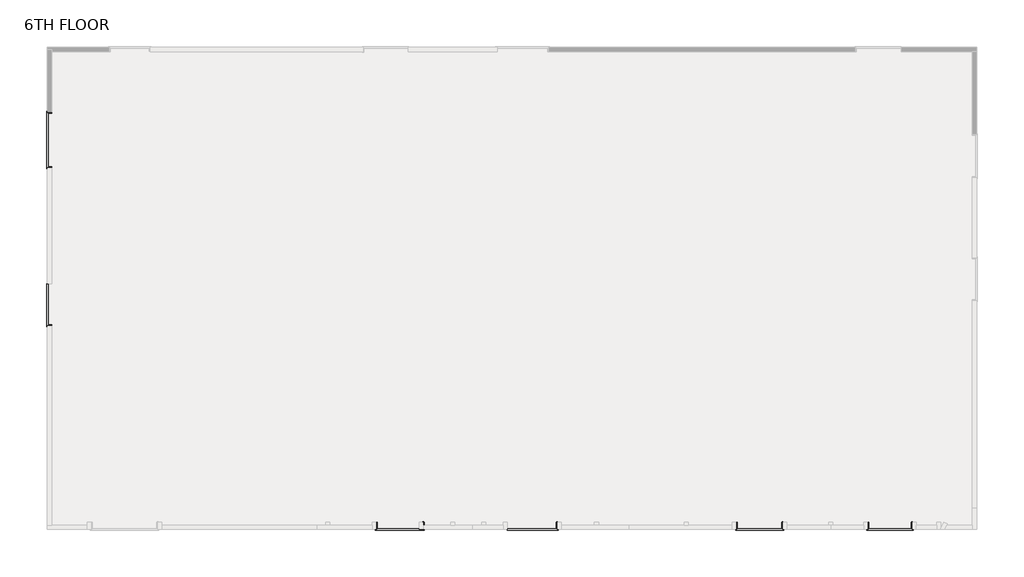
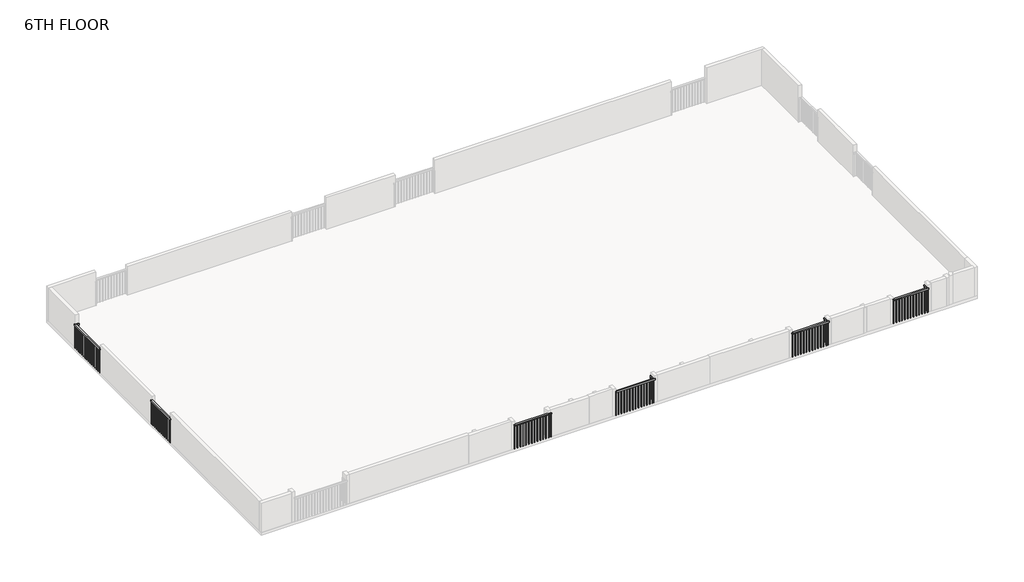
# One storey, part 2 of 3: 6 railings.
"""IFC4 building model written with IfcOpenShell, lengths in millimetres."""

from ifc_helpers import new_model, si_unit, frame, origin, place, context, project, spatial, polyline, outline, extrude, faceted_brep, element, save

model = new_model("IFC4")

# Units and contexts
model_context = context("Model", 3, world=origin())
ifc_project = project(units=[si_unit("LENGTHUNIT", "METRE", prefix="MILLI")], contexts=[model_context])

# Site, building, storey
site = spatial("IfcSite", under=ifc_project)
building = spatial("IfcBuilding", under=site)
storey = spatial("IfcBuildingStorey", under=building, Name="6TH FLOOR", Elevation=19202.4)

# Railings
placement = place(None, origin())
element("IfcRailing", 1, ObjectType="Handrail - Rectangular", at=placement, inside=storey, context=model_context, shape_type="SolidModel", body=[
    faceted_brep([(-3995.0987995, -4623.6932193, 20116.8), (-3995.0987995, -4623.6932193, 20066.0), (-4045.8987995, -4623.6932193, 20066.0), (-4045.8987995, -4623.6932193, 20116.8), (-3995.0987995, -4801.4932661, 20116.8), (-3995.0987995, -4801.4932661, 20066.0), (-4045.8987995, -4852.2932661, 20066.0), (-4045.8987995, -4852.2932661, 20116.8), (-2750.4987995, -4801.4932661, 20116.8), (-2750.4987995, -4801.4932661, 20066.0), (-2699.6987995, -4852.2932661, 20066.0), (-2699.6987995, -4852.2932661, 20116.8), (-2750.4987995, -4623.6932193, 20116.8), (-2699.6987995, -4623.6932193, 20116.8), (-2699.6987995, -4623.6932193, 20066.0), (-2750.4987995, -4623.6932193, 20066.0)], [[[0, 1, 2, 3]], [[1, 0, 4, 5]], [[2, 1, 5, 6]], [[3, 2, 6, 7]], [[0, 3, 7, 4]], [[5, 4, 8, 9]], [[6, 5, 9, 10]], [[7, 6, 10, 11]], [[4, 7, 11, 8]], [[12, 13, 14, 15]], [[9, 8, 12, 15]], [[10, 9, 15, 14]], [[11, 10, 14, 13]], [[8, 11, 13, 12]]]),
    extrude(outline(polyline([(-2715.5737995, -4633.2182661), (-2734.6237995, -4633.2182661), (-2734.6237995, -4614.1682661), (-2715.5737995, -4614.1682661), (-2715.5737995, -4633.2182661)])), frame((0.0, 0.0, 19202.4), z_axis=(0.0, 0.0, 1.0), x_axis=(1.0, 0.0, 0.0)), (0.0, 0.0, 1.0), 863.6),
    extrude(outline(polyline([(-2715.5737995, -4734.8182661), (-2734.6237995, -4734.8182661), (-2734.6237995, -4715.7682661), (-2715.5737995, -4715.7682661), (-2715.5737995, -4734.8182661)])), frame((0.0, 0.0, 19202.4), z_axis=(0.0, 0.0, 1.0), x_axis=(1.0, 0.0, 0.0)), (0.0, 0.0, 1.0), 863.6),
    extrude(outline(polyline([(-2810.8237995, -4836.4182661), (-2810.8237995, -4817.3682661), (-2791.7737995, -4817.3682661), (-2791.7737995, -4836.4182661), (-2810.8237995, -4836.4182661)])), frame((0.0, 0.0, 19202.4), z_axis=(0.0, 0.0, 1.0), x_axis=(1.0, 0.0, 0.0)), (0.0, 0.0, 1.0), 863.6),
    extrude(outline(polyline([(-2912.4237995, -4836.4182661), (-2912.4237995, -4817.3682661), (-2893.3737995, -4817.3682661), (-2893.3737995, -4836.4182661), (-2912.4237995, -4836.4182661)])), frame((0.0, 0.0, 19202.4), z_axis=(0.0, 0.0, 1.0), x_axis=(1.0, 0.0, 0.0)), (0.0, 0.0, 1.0), 863.6),
    extrude(outline(polyline([(-3014.0237995, -4836.4182661), (-3014.0237995, -4817.3682661), (-2994.9737995, -4817.3682661), (-2994.9737995, -4836.4182661), (-3014.0237995, -4836.4182661)])), frame((0.0, 0.0, 19202.4), z_axis=(0.0, 0.0, 1.0), x_axis=(1.0, 0.0, 0.0)), (0.0, 0.0, 1.0), 863.6),
    extrude(outline(polyline([(-3115.6237995, -4836.4182661), (-3115.6237995, -4817.3682661), (-3096.5737995, -4817.3682661), (-3096.5737995, -4836.4182661), (-3115.6237995, -4836.4182661)])), frame((0.0, 0.0, 19202.4), z_axis=(0.0, 0.0, 1.0), x_axis=(1.0, 0.0, 0.0)), (0.0, 0.0, 1.0), 863.6),
    extrude(outline(polyline([(-3217.2237995, -4836.4182661), (-3217.2237995, -4817.3682661), (-3198.1737995, -4817.3682661), (-3198.1737995, -4836.4182661), (-3217.2237995, -4836.4182661)])), frame((0.0, 0.0, 19202.4), z_axis=(0.0, 0.0, 1.0), x_axis=(1.0, 0.0, 0.0)), (0.0, 0.0, 1.0), 863.6),
    extrude(outline(polyline([(-3318.8237995, -4836.4182661), (-3318.8237995, -4817.3682661), (-3299.7737995, -4817.3682661), (-3299.7737995, -4836.4182661), (-3318.8237995, -4836.4182661)])), frame((0.0, 0.0, 19202.4), z_axis=(0.0, 0.0, 1.0), x_axis=(1.0, 0.0, 0.0)), (0.0, 0.0, 1.0), 863.6),
    extrude(outline(polyline([(-3420.4237995, -4836.4182661), (-3420.4237995, -4817.3682661), (-3401.3737995, -4817.3682661), (-3401.3737995, -4836.4182661), (-3420.4237995, -4836.4182661)])), frame((0.0, 0.0, 19202.4), z_axis=(0.0, 0.0, 1.0), x_axis=(1.0, 0.0, 0.0)), (0.0, 0.0, 1.0), 863.6),
    extrude(outline(polyline([(-3522.0237995, -4836.4182661), (-3522.0237995, -4817.3682661), (-3502.9737995, -4817.3682661), (-3502.9737995, -4836.4182661), (-3522.0237995, -4836.4182661)])), frame((0.0, 0.0, 19202.4), z_axis=(0.0, 0.0, 1.0), x_axis=(1.0, 0.0, 0.0)), (0.0, 0.0, 1.0), 863.6),
    extrude(outline(polyline([(-3623.6237995, -4836.4182661), (-3623.6237995, -4817.3682661), (-3604.5737995, -4817.3682661), (-3604.5737995, -4836.4182661), (-3623.6237995, -4836.4182661)])), frame((0.0, 0.0, 19202.4), z_axis=(0.0, 0.0, 1.0), x_axis=(1.0, 0.0, 0.0)), (0.0, 0.0, 1.0), 863.6),
    extrude(outline(polyline([(-3725.2237995, -4836.4182661), (-3725.2237995, -4817.3682661), (-3706.1737995, -4817.3682661), (-3706.1737995, -4836.4182661), (-3725.2237995, -4836.4182661)])), frame((0.0, 0.0, 19202.4), z_axis=(0.0, 0.0, 1.0), x_axis=(1.0, 0.0, 0.0)), (0.0, 0.0, 1.0), 863.6),
    extrude(outline(polyline([(-3826.8237995, -4836.4182661), (-3826.8237995, -4817.3682661), (-3807.7737995, -4817.3682661), (-3807.7737995, -4836.4182661), (-3826.8237995, -4836.4182661)])), frame((0.0, 0.0, 19202.4), z_axis=(0.0, 0.0, 1.0), x_axis=(1.0, 0.0, 0.0)), (0.0, 0.0, 1.0), 863.6),
    extrude(outline(polyline([(-3928.4237995, -4836.4182661), (-3928.4237995, -4817.3682661), (-3909.3737995, -4817.3682661), (-3909.3737995, -4836.4182661), (-3928.4237995, -4836.4182661)])), frame((0.0, 0.0, 19202.4), z_axis=(0.0, 0.0, 1.0), x_axis=(1.0, 0.0, 0.0)), (0.0, 0.0, 1.0), 863.6),
    extrude(outline(polyline([(-4030.0237995, -4817.3682193), (-4010.9737995, -4817.3682193), (-4010.9737995, -4836.4182193), (-4030.0237995, -4836.4182193), (-4030.0237995, -4817.3682193)])), frame((0.0, 0.0, 19202.4), z_axis=(0.0, 0.0, 1.0), x_axis=(1.0, 0.0, 0.0)), (0.0, 0.0, 1.0), 863.6),
    extrude(outline(polyline([(-4030.0237995, -4715.7682193), (-4010.9737995, -4715.7682193), (-4010.9737995, -4734.8182193), (-4030.0237995, -4734.8182193), (-4030.0237995, -4715.7682193)])), frame((0.0, 0.0, 19202.4), z_axis=(0.0, 0.0, 1.0), x_axis=(1.0, 0.0, 0.0)), (0.0, 0.0, 1.0), 863.6),
    extrude(outline(polyline([(-2734.6237995, -4836.4182661), (-2734.6237995, -4817.3682661), (-2715.5737995, -4817.3682661), (-2715.5737995, -4836.4182661), (-2734.6237995, -4836.4182661)])), frame((0.0, 0.0, 19202.4), z_axis=(0.0, 0.0, 1.0), x_axis=(1.0, 0.0, 0.0)), (0.0, 0.0, 1.0), 863.6),
    extrude(outline(polyline([(-4030.0237995, -4817.3682661), (-4010.9737995, -4817.3682661), (-4010.9737995, -4836.4182661), (-4030.0237995, -4836.4182661), (-4030.0237995, -4817.3682661)])), frame((0.0, 0.0, 19202.4), z_axis=(0.0, 0.0, 1.0), x_axis=(1.0, 0.0, 0.0)), (0.0, 0.0, 1.0), 863.6),
    extrude(outline(polyline([(-2715.5737995, -4642.7432193), (-2734.6237995, -4642.7432193), (-2734.6237995, -4623.6932193), (-2715.5737995, -4623.6932193), (-2715.5737995, -4642.7432193)])), frame((0.0, 0.0, 19202.4), z_axis=(0.0, 0.0, 1.0), x_axis=(1.0, 0.0, 0.0)), (0.0, 0.0, 1.0), 863.6),
    extrude(outline(polyline([(-4030.0237995, -4623.6932193), (-4010.9737995, -4623.6932193), (-4010.9737995, -4642.7432193), (-4030.0237995, -4642.7432193), (-4030.0237995, -4623.6932193)])), frame((0.0, 0.0, 19202.4), z_axis=(0.0, 0.0, 1.0), x_axis=(1.0, 0.0, 0.0)), (0.0, 0.0, 1.0), 863.6),
])
element("IfcRailing", 2, ObjectType="Handrail - Rectangular", at=placement, inside=storey, context=model_context, shape_type="SolidModel", body=[
    faceted_brep([(-406.2065315, -4801.4932661, 20116.8), (-406.2065315, -4801.4932661, 20066.0), (-406.2065315, -4852.2932661, 20066.0), (-406.2065315, -4852.2932661, 20116.8), (944.6932011, -4801.4932661, 20116.8), (944.6932011, -4801.4932661, 20066.0), (995.4932011, -4852.2932661, 20066.0), (995.4932011, -4852.2932661, 20116.8), (944.6932011, -4623.6932193, 20116.8), (995.4932011, -4623.6932193, 20116.8), (995.4932011, -4623.6932193, 20066.0), (944.6932011, -4623.6932193, 20066.0)], [[[0, 1, 2, 3]], [[1, 0, 4, 5]], [[2, 1, 5, 6]], [[3, 2, 6, 7]], [[0, 3, 7, 4]], [[8, 9, 10, 11]], [[5, 4, 8, 11]], [[6, 5, 11, 10]], [[7, 6, 10, 9]], [[4, 7, 9, 8]]]),
    extrude(outline(polyline([(979.6182011, -4633.2182661), (960.5682011, -4633.2182661), (960.5682011, -4614.1682661), (979.6182011, -4614.1682661), (979.6182011, -4633.2182661)])), frame((0.0, 0.0, 19202.4), z_axis=(0.0, 0.0, 1.0), x_axis=(1.0, 0.0, 0.0)), (0.0, 0.0, 1.0), 863.6),
    extrude(outline(polyline([(979.6182011, -4734.8182661), (960.5682011, -4734.8182661), (960.5682011, -4715.7682661), (979.6182011, -4715.7682661), (979.6182011, -4734.8182661)])), frame((0.0, 0.0, 19202.4), z_axis=(0.0, 0.0, 1.0), x_axis=(1.0, 0.0, 0.0)), (0.0, 0.0, 1.0), 863.6),
    extrude(outline(polyline([(905.0684685, -4836.4182661), (905.0684685, -4817.3682661), (924.1184685, -4817.3682661), (924.1184685, -4836.4182661), (905.0684685, -4836.4182661)])), frame((0.0, 0.0, 19202.4), z_axis=(0.0, 0.0, 1.0), x_axis=(1.0, 0.0, 0.0)), (0.0, 0.0, 1.0), 863.6),
    extrude(outline(polyline([(803.4684685, -4836.4182661), (803.4684685, -4817.3682661), (822.5184685, -4817.3682661), (822.5184685, -4836.4182661), (803.4684685, -4836.4182661)])), frame((0.0, 0.0, 19202.4), z_axis=(0.0, 0.0, 1.0), x_axis=(1.0, 0.0, 0.0)), (0.0, 0.0, 1.0), 863.6),
    extrude(outline(polyline([(701.8684685, -4836.4182661), (701.8684685, -4817.3682661), (720.9184685, -4817.3682661), (720.9184685, -4836.4182661), (701.8684685, -4836.4182661)])), frame((0.0, 0.0, 19202.4), z_axis=(0.0, 0.0, 1.0), x_axis=(1.0, 0.0, 0.0)), (0.0, 0.0, 1.0), 863.6),
    extrude(outline(polyline([(600.2684685, -4836.4182661), (600.2684685, -4817.3682661), (619.3184685, -4817.3682661), (619.3184685, -4836.4182661), (600.2684685, -4836.4182661)])), frame((0.0, 0.0, 19202.4), z_axis=(0.0, 0.0, 1.0), x_axis=(1.0, 0.0, 0.0)), (0.0, 0.0, 1.0), 863.6),
    extrude(outline(polyline([(498.6684685, -4836.4182661), (498.6684685, -4817.3682661), (517.7184685, -4817.3682661), (517.7184685, -4836.4182661), (498.6684685, -4836.4182661)])), frame((0.0, 0.0, 19202.4), z_axis=(0.0, 0.0, 1.0), x_axis=(1.0, 0.0, 0.0)), (0.0, 0.0, 1.0), 863.6),
    extrude(outline(polyline([(397.0684685, -4836.4182661), (397.0684685, -4817.3682661), (416.1184685, -4817.3682661), (416.1184685, -4836.4182661), (397.0684685, -4836.4182661)])), frame((0.0, 0.0, 19202.4), z_axis=(0.0, 0.0, 1.0), x_axis=(1.0, 0.0, 0.0)), (0.0, 0.0, 1.0), 863.6),
    extrude(outline(polyline([(295.4684685, -4836.4182661), (295.4684685, -4817.3682661), (314.5184685, -4817.3682661), (314.5184685, -4836.4182661), (295.4684685, -4836.4182661)])), frame((0.0, 0.0, 19202.4), z_axis=(0.0, 0.0, 1.0), x_axis=(1.0, 0.0, 0.0)), (0.0, 0.0, 1.0), 863.6),
    extrude(outline(polyline([(193.8684685, -4836.4182661), (193.8684685, -4817.3682661), (212.9184685, -4817.3682661), (212.9184685, -4836.4182661), (193.8684685, -4836.4182661)])), frame((0.0, 0.0, 19202.4), z_axis=(0.0, 0.0, 1.0), x_axis=(1.0, 0.0, 0.0)), (0.0, 0.0, 1.0), 863.6),
    extrude(outline(polyline([(92.2684685, -4836.4182661), (92.2684685, -4817.3682661), (111.3184685, -4817.3682661), (111.3184685, -4836.4182661), (92.2684685, -4836.4182661)])), frame((0.0, 0.0, 19202.4), z_axis=(0.0, 0.0, 1.0), x_axis=(1.0, 0.0, 0.0)), (0.0, 0.0, 1.0), 863.6),
    extrude(outline(polyline([(-9.3315315, -4836.4182661), (-9.3315315, -4817.3682661), (9.7184685, -4817.3682661), (9.7184685, -4836.4182661), (-9.3315315, -4836.4182661)])), frame((0.0, 0.0, 19202.4), z_axis=(0.0, 0.0, 1.0), x_axis=(1.0, 0.0, 0.0)), (0.0, 0.0, 1.0), 863.6),
    extrude(outline(polyline([(-110.9315315, -4836.4182661), (-110.9315315, -4817.3682661), (-91.8815315, -4817.3682661), (-91.8815315, -4836.4182661), (-110.9315315, -4836.4182661)])), frame((0.0, 0.0, 19202.4), z_axis=(0.0, 0.0, 1.0), x_axis=(1.0, 0.0, 0.0)), (0.0, 0.0, 1.0), 863.6),
    extrude(outline(polyline([(-212.5315315, -4836.4182661), (-212.5315315, -4817.3682661), (-193.4815315, -4817.3682661), (-193.4815315, -4836.4182661), (-212.5315315, -4836.4182661)])), frame((0.0, 0.0, 19202.4), z_axis=(0.0, 0.0, 1.0), x_axis=(1.0, 0.0, 0.0)), (0.0, 0.0, 1.0), 863.6),
    extrude(outline(polyline([(-314.1315315, -4836.4182661), (-314.1315315, -4817.3682661), (-295.0815315, -4817.3682661), (-295.0815315, -4836.4182661), (-314.1315315, -4836.4182661)])), frame((0.0, 0.0, 19202.4), z_axis=(0.0, 0.0, 1.0), x_axis=(1.0, 0.0, 0.0)), (0.0, 0.0, 1.0), 863.6),
    extrude(outline(polyline([(960.5682011, -4836.4182661), (960.5682011, -4817.3682661), (979.6182011, -4817.3682661), (979.6182011, -4836.4182661), (960.5682011, -4836.4182661)])), frame((0.0, 0.0, 19202.4), z_axis=(0.0, 0.0, 1.0), x_axis=(1.0, 0.0, 0.0)), (0.0, 0.0, 1.0), 863.6),
    extrude(outline(polyline([(979.6182011, -4642.7432193), (960.5682011, -4642.7432193), (960.5682011, -4623.6932193), (979.6182011, -4623.6932193), (979.6182011, -4642.7432193)])), frame((0.0, 0.0, 19202.4), z_axis=(0.0, 0.0, 1.0), x_axis=(1.0, 0.0, 0.0)), (0.0, 0.0, 1.0), 863.6),
    extrude(outline(polyline([(-406.2065315, -4836.4182661), (-406.2065315, -4817.3682661), (-387.1565315, -4817.3682661), (-387.1565315, -4836.4182661), (-406.2065315, -4836.4182661)])), frame((0.0, 0.0, 19202.4), z_axis=(0.0, 0.0, 1.0), x_axis=(1.0, 0.0, 0.0)), (0.0, 0.0, 1.0), 863.6),
])
element("IfcRailing", 3, ObjectType="Handrail - Rectangular", at=placement, inside=storey, context=model_context, shape_type="SolidModel", body=[
    faceted_brep([(5942.6512082, -4623.6932193, 20116.8), (5942.6512082, -4623.6932193, 20066.0), (5891.8512082, -4623.6932193, 20066.0), (5891.8512082, -4623.6932193, 20116.8), (5942.6512082, -4801.4932661, 20116.8), (5942.6512082, -4801.4932661, 20066.0), (5891.8512082, -4852.2932661, 20066.0), (5891.8512082, -4852.2932661, 20116.8), (7164.9011643, -4801.4932661, 20116.8), (7164.9011643, -4801.4932661, 20066.0), (7215.7011643, -4852.2932661, 20066.0), (7215.7011643, -4852.2932661, 20116.8), (7164.9011643, -4623.6932193, 20116.8), (7215.7011643, -4623.6932193, 20116.8), (7215.7011643, -4623.6932193, 20066.0), (7164.9011643, -4623.6932193, 20066.0)], [[[0, 1, 2, 3]], [[1, 0, 4, 5]], [[2, 1, 5, 6]], [[3, 2, 6, 7]], [[0, 3, 7, 4]], [[5, 4, 8, 9]], [[6, 5, 9, 10]], [[7, 6, 10, 11]], [[4, 7, 11, 8]], [[12, 13, 14, 15]], [[9, 8, 12, 15]], [[10, 9, 15, 14]], [[11, 10, 14, 13]], [[8, 11, 13, 12]]]),
    extrude(outline(polyline([(7199.8261643, -4633.2182661), (7180.7761643, -4633.2182661), (7180.7761643, -4614.1682661), (7199.8261643, -4614.1682661), (7199.8261643, -4633.2182661)])), frame((0.0, 0.0, 19202.4), z_axis=(0.0, 0.0, 1.0), x_axis=(1.0, 0.0, 0.0)), (0.0, 0.0, 1.0), 863.6),
    extrude(outline(polyline([(7199.8261643, -4734.8182661), (7180.7761643, -4734.8182661), (7180.7761643, -4715.7682661), (7199.8261643, -4715.7682661), (7199.8261643, -4734.8182661)])), frame((0.0, 0.0, 19202.4), z_axis=(0.0, 0.0, 1.0), x_axis=(1.0, 0.0, 0.0)), (0.0, 0.0, 1.0), 863.6),
    extrude(outline(polyline([(7126.9262082, -4836.4182661), (7126.9262082, -4817.3682661), (7145.9762082, -4817.3682661), (7145.9762082, -4836.4182661), (7126.9262082, -4836.4182661)])), frame((0.0, 0.0, 19202.4), z_axis=(0.0, 0.0, 1.0), x_axis=(1.0, 0.0, 0.0)), (0.0, 0.0, 1.0), 863.6),
    extrude(outline(polyline([(7025.3262082, -4836.4182661), (7025.3262082, -4817.3682661), (7044.3762082, -4817.3682661), (7044.3762082, -4836.4182661), (7025.3262082, -4836.4182661)])), frame((0.0, 0.0, 19202.4), z_axis=(0.0, 0.0, 1.0), x_axis=(1.0, 0.0, 0.0)), (0.0, 0.0, 1.0), 863.6),
    extrude(outline(polyline([(6923.7262082, -4836.4182661), (6923.7262082, -4817.3682661), (6942.7762082, -4817.3682661), (6942.7762082, -4836.4182661), (6923.7262082, -4836.4182661)])), frame((0.0, 0.0, 19202.4), z_axis=(0.0, 0.0, 1.0), x_axis=(1.0, 0.0, 0.0)), (0.0, 0.0, 1.0), 863.6),
    extrude(outline(polyline([(6822.1262082, -4836.4182661), (6822.1262082, -4817.3682661), (6841.1762082, -4817.3682661), (6841.1762082, -4836.4182661), (6822.1262082, -4836.4182661)])), frame((0.0, 0.0, 19202.4), z_axis=(0.0, 0.0, 1.0), x_axis=(1.0, 0.0, 0.0)), (0.0, 0.0, 1.0), 863.6),
    extrude(outline(polyline([(6720.5262082, -4836.4182661), (6720.5262082, -4817.3682661), (6739.5762082, -4817.3682661), (6739.5762082, -4836.4182661), (6720.5262082, -4836.4182661)])), frame((0.0, 0.0, 19202.4), z_axis=(0.0, 0.0, 1.0), x_axis=(1.0, 0.0, 0.0)), (0.0, 0.0, 1.0), 863.6),
    extrude(outline(polyline([(6618.9262082, -4836.4182661), (6618.9262082, -4817.3682661), (6637.9762082, -4817.3682661), (6637.9762082, -4836.4182661), (6618.9262082, -4836.4182661)])), frame((0.0, 0.0, 19202.4), z_axis=(0.0, 0.0, 1.0), x_axis=(1.0, 0.0, 0.0)), (0.0, 0.0, 1.0), 863.6),
    extrude(outline(polyline([(6517.3262082, -4836.4182661), (6517.3262082, -4817.3682661), (6536.3762082, -4817.3682661), (6536.3762082, -4836.4182661), (6517.3262082, -4836.4182661)])), frame((0.0, 0.0, 19202.4), z_axis=(0.0, 0.0, 1.0), x_axis=(1.0, 0.0, 0.0)), (0.0, 0.0, 1.0), 863.6),
    extrude(outline(polyline([(6415.7262082, -4836.4182661), (6415.7262082, -4817.3682661), (6434.7762082, -4817.3682661), (6434.7762082, -4836.4182661), (6415.7262082, -4836.4182661)])), frame((0.0, 0.0, 19202.4), z_axis=(0.0, 0.0, 1.0), x_axis=(1.0, 0.0, 0.0)), (0.0, 0.0, 1.0), 863.6),
    extrude(outline(polyline([(6314.1262082, -4836.4182661), (6314.1262082, -4817.3682661), (6333.1762082, -4817.3682661), (6333.1762082, -4836.4182661), (6314.1262082, -4836.4182661)])), frame((0.0, 0.0, 19202.4), z_axis=(0.0, 0.0, 1.0), x_axis=(1.0, 0.0, 0.0)), (0.0, 0.0, 1.0), 863.6),
    extrude(outline(polyline([(6212.5262082, -4836.4182661), (6212.5262082, -4817.3682661), (6231.5762082, -4817.3682661), (6231.5762082, -4836.4182661), (6212.5262082, -4836.4182661)])), frame((0.0, 0.0, 19202.4), z_axis=(0.0, 0.0, 1.0), x_axis=(1.0, 0.0, 0.0)), (0.0, 0.0, 1.0), 863.6),
    extrude(outline(polyline([(6110.9262082, -4836.4182661), (6110.9262082, -4817.3682661), (6129.9762082, -4817.3682661), (6129.9762082, -4836.4182661), (6110.9262082, -4836.4182661)])), frame((0.0, 0.0, 19202.4), z_axis=(0.0, 0.0, 1.0), x_axis=(1.0, 0.0, 0.0)), (0.0, 0.0, 1.0), 863.6),
    extrude(outline(polyline([(6009.3262082, -4836.4182661), (6009.3262082, -4817.3682661), (6028.3762082, -4817.3682661), (6028.3762082, -4836.4182661), (6009.3262082, -4836.4182661)])), frame((0.0, 0.0, 19202.4), z_axis=(0.0, 0.0, 1.0), x_axis=(1.0, 0.0, 0.0)), (0.0, 0.0, 1.0), 863.6),
    extrude(outline(polyline([(5907.7262082, -4817.3682193), (5926.7762082, -4817.3682193), (5926.7762082, -4836.4182193), (5907.7262082, -4836.4182193), (5907.7262082, -4817.3682193)])), frame((0.0, 0.0, 19202.4), z_axis=(0.0, 0.0, 1.0), x_axis=(1.0, 0.0, 0.0)), (0.0, 0.0, 1.0), 863.6),
    extrude(outline(polyline([(5907.7262082, -4715.7682193), (5926.7762082, -4715.7682193), (5926.7762082, -4734.8182193), (5907.7262082, -4734.8182193), (5907.7262082, -4715.7682193)])), frame((0.0, 0.0, 19202.4), z_axis=(0.0, 0.0, 1.0), x_axis=(1.0, 0.0, 0.0)), (0.0, 0.0, 1.0), 863.6),
    extrude(outline(polyline([(7180.7761643, -4836.4182661), (7180.7761643, -4817.3682661), (7199.8261643, -4817.3682661), (7199.8261643, -4836.4182661), (7180.7761643, -4836.4182661)])), frame((0.0, 0.0, 19202.4), z_axis=(0.0, 0.0, 1.0), x_axis=(1.0, 0.0, 0.0)), (0.0, 0.0, 1.0), 863.6),
    extrude(outline(polyline([(5907.7262082, -4817.3682661), (5926.7762082, -4817.3682661), (5926.7762082, -4836.4182661), (5907.7262082, -4836.4182661), (5907.7262082, -4817.3682661)])), frame((0.0, 0.0, 19202.4), z_axis=(0.0, 0.0, 1.0), x_axis=(1.0, 0.0, 0.0)), (0.0, 0.0, 1.0), 863.6),
    extrude(outline(polyline([(7199.8261643, -4642.7432193), (7180.7761643, -4642.7432193), (7180.7761643, -4623.6932193), (7199.8261643, -4623.6932193), (7199.8261643, -4642.7432193)])), frame((0.0, 0.0, 19202.4), z_axis=(0.0, 0.0, 1.0), x_axis=(1.0, 0.0, 0.0)), (0.0, 0.0, 1.0), 863.6),
    extrude(outline(polyline([(5907.7262082, -4623.6932193), (5926.7762082, -4623.6932193), (5926.7762082, -4642.7432193), (5907.7262082, -4642.7432193), (5907.7262082, -4623.6932193)])), frame((0.0, 0.0, 19202.4), z_axis=(0.0, 0.0, 1.0), x_axis=(1.0, 0.0, 0.0)), (0.0, 0.0, 1.0), 863.6),
])
element("IfcRailing", 4, ObjectType="Handrail - Rectangular", at=placement, inside=storey, context=model_context, shape_type="SolidModel", body=[
    faceted_brep([(9562.1512082, -4623.6932193, 20116.8), (9562.1512082, -4623.6932193, 20066.0), (9511.3512082, -4623.6932193, 20066.0), (9511.3512082, -4623.6932193, 20116.8), (9562.1512082, -4801.4932661, 20116.8), (9562.1512082, -4801.4932661, 20066.0), (9511.3512082, -4852.2932661, 20066.0), (9511.3512082, -4852.2932661, 20116.8), (10738.7617205, -4801.4932661, 20116.8), (10738.7617205, -4801.4932661, 20066.0), (10789.5617205, -4852.2932661, 20066.0), (10789.5617205, -4852.2932661, 20116.8), (10738.7617205, -4623.6932193, 20116.8), (10789.5617205, -4623.6932193, 20116.8), (10789.5617205, -4623.6932193, 20066.0), (10738.7617205, -4623.6932193, 20066.0)], [[[0, 1, 2, 3]], [[1, 0, 4, 5]], [[2, 1, 5, 6]], [[3, 2, 6, 7]], [[0, 3, 7, 4]], [[5, 4, 8, 9]], [[6, 5, 9, 10]], [[7, 6, 10, 11]], [[4, 7, 11, 8]], [[12, 13, 14, 15]], [[9, 8, 12, 15]], [[10, 9, 15, 14]], [[11, 10, 14, 13]], [[8, 11, 13, 12]]]),
    extrude(outline(polyline([(10754.6367205, -4633.2182661), (10754.6367205, -4614.1682661), (10773.6867205, -4614.1682661), (10773.6867205, -4633.2182661), (10754.6367205, -4633.2182661)])), frame((0.0, 0.0, 19202.4), z_axis=(0.0, 0.0, 1.0), x_axis=(1.0, 0.0, 0.0)), (0.0, 0.0, 1.0), 863.6),
    extrude(outline(polyline([(10754.6367205, -4734.8182661), (10754.6367205, -4715.7682661), (10773.6867205, -4715.7682661), (10773.6867205, -4734.8182661), (10754.6367205, -4734.8182661)])), frame((0.0, 0.0, 19202.4), z_axis=(0.0, 0.0, 1.0), x_axis=(1.0, 0.0, 0.0)), (0.0, 0.0, 1.0), 863.6),
    extrude(outline(polyline([(10746.4262082, -4817.3682661), (10765.4762082, -4817.3682661), (10765.4762082, -4836.4182661), (10746.4262082, -4836.4182661), (10746.4262082, -4817.3682661)])), frame((0.0, 0.0, 19202.4), z_axis=(0.0, 0.0, 1.0), x_axis=(1.0, 0.0, 0.0)), (0.0, 0.0, 1.0), 863.6),
    extrude(outline(polyline([(10644.8262082, -4817.3682661), (10663.8762082, -4817.3682661), (10663.8762082, -4836.4182661), (10644.8262082, -4836.4182661), (10644.8262082, -4817.3682661)])), frame((0.0, 0.0, 19202.4), z_axis=(0.0, 0.0, 1.0), x_axis=(1.0, 0.0, 0.0)), (0.0, 0.0, 1.0), 863.6),
    extrude(outline(polyline([(10543.2262082, -4817.3682661), (10562.2762082, -4817.3682661), (10562.2762082, -4836.4182661), (10543.2262082, -4836.4182661), (10543.2262082, -4817.3682661)])), frame((0.0, 0.0, 19202.4), z_axis=(0.0, 0.0, 1.0), x_axis=(1.0, 0.0, 0.0)), (0.0, 0.0, 1.0), 863.6),
    extrude(outline(polyline([(10441.6262082, -4817.3682661), (10460.6762082, -4817.3682661), (10460.6762082, -4836.4182661), (10441.6262082, -4836.4182661), (10441.6262082, -4817.3682661)])), frame((0.0, 0.0, 19202.4), z_axis=(0.0, 0.0, 1.0), x_axis=(1.0, 0.0, 0.0)), (0.0, 0.0, 1.0), 863.6),
    extrude(outline(polyline([(10340.0262082, -4817.3682661), (10359.0762082, -4817.3682661), (10359.0762082, -4836.4182661), (10340.0262082, -4836.4182661), (10340.0262082, -4817.3682661)])), frame((0.0, 0.0, 19202.4), z_axis=(0.0, 0.0, 1.0), x_axis=(1.0, 0.0, 0.0)), (0.0, 0.0, 1.0), 863.6),
    extrude(outline(polyline([(10238.4262082, -4817.3682661), (10257.4762082, -4817.3682661), (10257.4762082, -4836.4182661), (10238.4262082, -4836.4182661), (10238.4262082, -4817.3682661)])), frame((0.0, 0.0, 19202.4), z_axis=(0.0, 0.0, 1.0), x_axis=(1.0, 0.0, 0.0)), (0.0, 0.0, 1.0), 863.6),
    extrude(outline(polyline([(10136.8262082, -4817.3682661), (10155.8762082, -4817.3682661), (10155.8762082, -4836.4182661), (10136.8262082, -4836.4182661), (10136.8262082, -4817.3682661)])), frame((0.0, 0.0, 19202.4), z_axis=(0.0, 0.0, 1.0), x_axis=(1.0, 0.0, 0.0)), (0.0, 0.0, 1.0), 863.6),
    extrude(outline(polyline([(10035.2262082, -4817.3682661), (10054.2762082, -4817.3682661), (10054.2762082, -4836.4182661), (10035.2262082, -4836.4182661), (10035.2262082, -4817.3682661)])), frame((0.0, 0.0, 19202.4), z_axis=(0.0, 0.0, 1.0), x_axis=(1.0, 0.0, 0.0)), (0.0, 0.0, 1.0), 863.6),
    extrude(outline(polyline([(9933.6262082, -4817.3682661), (9952.6762082, -4817.3682661), (9952.6762082, -4836.4182661), (9933.6262082, -4836.4182661), (9933.6262082, -4817.3682661)])), frame((0.0, 0.0, 19202.4), z_axis=(0.0, 0.0, 1.0), x_axis=(1.0, 0.0, 0.0)), (0.0, 0.0, 1.0), 863.6),
    extrude(outline(polyline([(9832.0262082, -4817.3682661), (9851.0762082, -4817.3682661), (9851.0762082, -4836.4182661), (9832.0262082, -4836.4182661), (9832.0262082, -4817.3682661)])), frame((0.0, 0.0, 19202.4), z_axis=(0.0, 0.0, 1.0), x_axis=(1.0, 0.0, 0.0)), (0.0, 0.0, 1.0), 863.6),
    extrude(outline(polyline([(9730.4262082, -4817.3682661), (9749.4762082, -4817.3682661), (9749.4762082, -4836.4182661), (9730.4262082, -4836.4182661), (9730.4262082, -4817.3682661)])), frame((0.0, 0.0, 19202.4), z_axis=(0.0, 0.0, 1.0), x_axis=(1.0, 0.0, 0.0)), (0.0, 0.0, 1.0), 863.6),
    extrude(outline(polyline([(9628.8262082, -4817.3682661), (9647.8762082, -4817.3682661), (9647.8762082, -4836.4182661), (9628.8262082, -4836.4182661), (9628.8262082, -4817.3682661)])), frame((0.0, 0.0, 19202.4), z_axis=(0.0, 0.0, 1.0), x_axis=(1.0, 0.0, 0.0)), (0.0, 0.0, 1.0), 863.6),
    extrude(outline(polyline([(9546.2762082, -4817.3682193), (9546.2762082, -4836.4182193), (9527.2262082, -4836.4182193), (9527.2262082, -4817.3682193), (9546.2762082, -4817.3682193)])), frame((0.0, 0.0, 19202.4), z_axis=(0.0, 0.0, 1.0), x_axis=(1.0, 0.0, 0.0)), (0.0, 0.0, 1.0), 863.6),
    extrude(outline(polyline([(9546.2762082, -4715.7682193), (9546.2762082, -4734.8182193), (9527.2262082, -4734.8182193), (9527.2262082, -4715.7682193), (9546.2762082, -4715.7682193)])), frame((0.0, 0.0, 19202.4), z_axis=(0.0, 0.0, 1.0), x_axis=(1.0, 0.0, 0.0)), (0.0, 0.0, 1.0), 863.6),
    extrude(outline(polyline([(10754.6367205, -4817.3682661), (10773.6867205, -4817.3682661), (10773.6867205, -4836.4182661), (10754.6367205, -4836.4182661), (10754.6367205, -4817.3682661)])), frame((0.0, 0.0, 19202.4), z_axis=(0.0, 0.0, 1.0), x_axis=(1.0, 0.0, 0.0)), (0.0, 0.0, 1.0), 863.6),
    extrude(outline(polyline([(9546.2762082, -4817.3682661), (9546.2762082, -4836.4182661), (9527.2262082, -4836.4182661), (9527.2262082, -4817.3682661), (9546.2762082, -4817.3682661)])), frame((0.0, 0.0, 19202.4), z_axis=(0.0, 0.0, 1.0), x_axis=(1.0, 0.0, 0.0)), (0.0, 0.0, 1.0), 863.6),
    extrude(outline(polyline([(10754.6367205, -4642.7432193), (10754.6367205, -4623.6932193), (10773.6867205, -4623.6932193), (10773.6867205, -4642.7432193), (10754.6367205, -4642.7432193)])), frame((0.0, 0.0, 19202.4), z_axis=(0.0, 0.0, 1.0), x_axis=(1.0, 0.0, 0.0)), (0.0, 0.0, 1.0), 863.6),
    extrude(outline(polyline([(9546.2762082, -4623.6932193), (9546.2762082, -4642.7432193), (9527.2262082, -4642.7432193), (9527.2262082, -4623.6932193), (9546.2762082, -4623.6932193)])), frame((0.0, 0.0, 19202.4), z_axis=(0.0, 0.0, 1.0), x_axis=(1.0, 0.0, 0.0)), (0.0, 0.0, 1.0), 863.6),
])
element("IfcRailing", 5, ObjectType="Handrail - Rectangular", at=placement, inside=storey, context=model_context, shape_type="SolidModel", body=[
    faceted_brep([(-13063.4067989, 1953.9604213, 20116.8), (-13063.4067989, 1953.9604213, 20066.0), (-13114.2067989, 1953.9604213, 20066.0), (-13114.2067989, 1953.9604213, 20116.8), (-13063.4067989, 818.2567339, 20116.8), (-13063.4067989, 818.2567339, 20066.0), (-13114.2067989, 767.4567339, 20066.0), (-13114.2067989, 767.4567339, 20116.8), (-12974.5067989, 818.2567339, 20116.8), (-12974.5067989, 767.4567339, 20116.8), (-12974.5067989, 767.4567339, 20066.0), (-12974.5067989, 818.2567339, 20066.0)], [[[0, 1, 2, 3]], [[1, 0, 4, 5]], [[2, 1, 5, 6]], [[3, 2, 6, 7]], [[0, 3, 7, 4]], [[8, 9, 10, 11]], [[5, 4, 8, 11]], [[6, 5, 11, 10]], [[7, 6, 10, 9]], [[4, 7, 9, 8]]]),
    extrude(outline(polyline([(-12996.7317989, 783.3317339), (-12996.7317989, 802.3817339), (-12977.6817989, 802.3817339), (-12977.6817989, 783.3317339), (-12996.7317989, 783.3317339)])), frame((0.0, 0.0, 19202.4), z_axis=(0.0, 0.0, 1.0), x_axis=(1.0, 0.0, 0.0)), (0.0, 0.0, 1.0), 863.6),
    extrude(outline(polyline([(-13098.3317989, 845.8854213), (-13079.2817989, 845.8854213), (-13079.2817989, 826.8354213), (-13098.3317989, 826.8354213), (-13098.3317989, 845.8854213)])), frame((0.0, 0.0, 19202.4), z_axis=(0.0, 0.0, 1.0), x_axis=(1.0, 0.0, 0.0)), (0.0, 0.0, 1.0), 863.6),
    extrude(outline(polyline([(-13098.3317989, 947.4854213), (-13079.2817989, 947.4854213), (-13079.2817989, 928.4354213), (-13098.3317989, 928.4354213), (-13098.3317989, 947.4854213)])), frame((0.0, 0.0, 19202.4), z_axis=(0.0, 0.0, 1.0), x_axis=(1.0, 0.0, 0.0)), (0.0, 0.0, 1.0), 863.6),
    extrude(outline(polyline([(-13098.3317989, 1049.0854213), (-13079.2817989, 1049.0854213), (-13079.2817989, 1030.0354213), (-13098.3317989, 1030.0354213), (-13098.3317989, 1049.0854213)])), frame((0.0, 0.0, 19202.4), z_axis=(0.0, 0.0, 1.0), x_axis=(1.0, 0.0, 0.0)), (0.0, 0.0, 1.0), 863.6),
    extrude(outline(polyline([(-13098.3317989, 1150.6854213), (-13079.2817989, 1150.6854213), (-13079.2817989, 1131.6354213), (-13098.3317989, 1131.6354213), (-13098.3317989, 1150.6854213)])), frame((0.0, 0.0, 19202.4), z_axis=(0.0, 0.0, 1.0), x_axis=(1.0, 0.0, 0.0)), (0.0, 0.0, 1.0), 863.6),
    extrude(outline(polyline([(-13098.3317989, 1252.2854213), (-13079.2817989, 1252.2854213), (-13079.2817989, 1233.2354213), (-13098.3317989, 1233.2354213), (-13098.3317989, 1252.2854213)])), frame((0.0, 0.0, 19202.4), z_axis=(0.0, 0.0, 1.0), x_axis=(1.0, 0.0, 0.0)), (0.0, 0.0, 1.0), 863.6),
    extrude(outline(polyline([(-13098.3317989, 1353.8854213), (-13079.2817989, 1353.8854213), (-13079.2817989, 1334.8354213), (-13098.3317989, 1334.8354213), (-13098.3317989, 1353.8854213)])), frame((0.0, 0.0, 19202.4), z_axis=(0.0, 0.0, 1.0), x_axis=(1.0, 0.0, 0.0)), (0.0, 0.0, 1.0), 863.6),
    extrude(outline(polyline([(-13098.3317989, 1455.4854213), (-13079.2817989, 1455.4854213), (-13079.2817989, 1436.4354213), (-13098.3317989, 1436.4354213), (-13098.3317989, 1455.4854213)])), frame((0.0, 0.0, 19202.4), z_axis=(0.0, 0.0, 1.0), x_axis=(1.0, 0.0, 0.0)), (0.0, 0.0, 1.0), 863.6),
    extrude(outline(polyline([(-13098.3317989, 1557.0854213), (-13079.2817989, 1557.0854213), (-13079.2817989, 1538.0354213), (-13098.3317989, 1538.0354213), (-13098.3317989, 1557.0854213)])), frame((0.0, 0.0, 19202.4), z_axis=(0.0, 0.0, 1.0), x_axis=(1.0, 0.0, 0.0)), (0.0, 0.0, 1.0), 863.6),
    extrude(outline(polyline([(-13098.3317989, 1658.6854213), (-13079.2817989, 1658.6854213), (-13079.2817989, 1639.6354213), (-13098.3317989, 1639.6354213), (-13098.3317989, 1658.6854213)])), frame((0.0, 0.0, 19202.4), z_axis=(0.0, 0.0, 1.0), x_axis=(1.0, 0.0, 0.0)), (0.0, 0.0, 1.0), 863.6),
    extrude(outline(polyline([(-13098.3317989, 1760.2854213), (-13079.2817989, 1760.2854213), (-13079.2817989, 1741.2354213), (-13098.3317989, 1741.2354213), (-13098.3317989, 1760.2854213)])), frame((0.0, 0.0, 19202.4), z_axis=(0.0, 0.0, 1.0), x_axis=(1.0, 0.0, 0.0)), (0.0, 0.0, 1.0), 863.6),
    extrude(outline(polyline([(-13098.3317989, 1861.8854213), (-13079.2817989, 1861.8854213), (-13079.2817989, 1842.8354213), (-13098.3317989, 1842.8354213), (-13098.3317989, 1861.8854213)])), frame((0.0, 0.0, 19202.4), z_axis=(0.0, 0.0, 1.0), x_axis=(1.0, 0.0, 0.0)), (0.0, 0.0, 1.0), 863.6),
    extrude(outline(polyline([(-13098.3317989, 802.3817339), (-13079.2817989, 802.3817339), (-13079.2817989, 783.3317339), (-13098.3317989, 783.3317339), (-13098.3317989, 802.3817339)])), frame((0.0, 0.0, 19202.4), z_axis=(0.0, 0.0, 1.0), x_axis=(1.0, 0.0, 0.0)), (0.0, 0.0, 1.0), 863.6),
    extrude(outline(polyline([(-13079.2817989, 1963.4854213), (-13079.2817989, 1944.4354213), (-13098.3317989, 1944.4354213), (-13098.3317989, 1963.4854213), (-13079.2817989, 1963.4854213)])), frame((0.0, 0.0, 19202.4), z_axis=(0.0, 0.0, 1.0), x_axis=(1.0, 0.0, 0.0)), (0.0, 0.0, 1.0), 863.6),
    extrude(outline(polyline([(-12993.5567989, 783.3317339), (-12993.5567989, 802.3817339), (-12974.5067989, 802.3817339), (-12974.5067989, 783.3317339), (-12993.5567989, 783.3317339)])), frame((0.0, 0.0, 19202.4), z_axis=(0.0, 0.0, 1.0), x_axis=(1.0, 0.0, 0.0)), (0.0, 0.0, 1.0), 863.6),
    extrude(outline(polyline([(-13062.8987925, 1963.4854213), (-13062.8987925, 1944.4354213), (-13081.9487925, 1944.4354213), (-13081.9487925, 1963.4854213), (-13062.8987925, 1963.4854213)])), frame((0.0, 0.0, 19202.4), z_axis=(0.0, 0.0, 1.0), x_axis=(1.0, 0.0, 0.0)), (0.0, 0.0, 1.0), 863.6),
])
element("IfcRailing", 6, ObjectType="Handrail - Rectangular", at=placement, inside=storey, context=model_context, shape_type="SolidModel", body=[
    faceted_brep([(-12973.9987925, 6656.8711337, 20116.8), (-12973.9987925, 6656.8711337, 20066.0), (-12973.9987925, 6707.6711337, 20066.0), (-12973.9987925, 6707.6711337, 20116.8), (-13062.8987925, 6656.8711337, 20116.8), (-13062.8987925, 6656.8711337, 20066.0), (-13113.6987925, 6707.6711337, 20066.0), (-13113.6987925, 6707.6711337, 20116.8), (-13062.8987925, 5180.1736362, 20116.8), (-13062.8987925, 5180.1736362, 20066.0), (-13113.6987925, 5129.3736362, 20066.0), (-13113.6987925, 5129.3736362, 20116.8), (-12973.9987925, 5180.1736362, 20116.8), (-12973.9987925, 5129.3736362, 20116.8), (-12973.9987925, 5129.3736362, 20066.0), (-12973.9987925, 5180.1736362, 20066.0)], [[[0, 1, 2, 3]], [[1, 0, 4, 5]], [[2, 1, 5, 6]], [[3, 2, 6, 7]], [[0, 3, 7, 4]], [[5, 4, 8, 9]], [[6, 5, 9, 10]], [[7, 6, 10, 11]], [[4, 7, 11, 8]], [[12, 13, 14, 15]], [[9, 8, 12, 15]], [[10, 9, 15, 14]], [[11, 10, 14, 13]], [[8, 11, 13, 12]]]),
    extrude(outline(polyline([(-12996.2237925, 5145.2486362), (-12996.2237925, 5164.2986362), (-12977.1737925, 5164.2986362), (-12977.1737925, 5145.2486362), (-12996.2237925, 5145.2486362)])), frame((0.0, 0.0, 19202.4), z_axis=(0.0, 0.0, 1.0), x_axis=(1.0, 0.0, 0.0)), (0.0, 0.0, 1.0), 863.6),
    extrude(outline(polyline([(-13097.8237925, 5167.7961337), (-13078.7737925, 5167.7961337), (-13078.7737925, 5148.7461337), (-13097.8237925, 5148.7461337), (-13097.8237925, 5167.7961337)])), frame((0.0, 0.0, 19202.4), z_axis=(0.0, 0.0, 1.0), x_axis=(1.0, 0.0, 0.0)), (0.0, 0.0, 1.0), 863.6),
    extrude(outline(polyline([(-13097.8237925, 5269.3961337), (-13078.7737925, 5269.3961337), (-13078.7737925, 5250.3461337), (-13097.8237925, 5250.3461337), (-13097.8237925, 5269.3961337)])), frame((0.0, 0.0, 19202.4), z_axis=(0.0, 0.0, 1.0), x_axis=(1.0, 0.0, 0.0)), (0.0, 0.0, 1.0), 863.6),
    extrude(outline(polyline([(-13097.8237925, 5370.9961337), (-13078.7737925, 5370.9961337), (-13078.7737925, 5351.9461337), (-13097.8237925, 5351.9461337), (-13097.8237925, 5370.9961337)])), frame((0.0, 0.0, 19202.4), z_axis=(0.0, 0.0, 1.0), x_axis=(1.0, 0.0, 0.0)), (0.0, 0.0, 1.0), 863.6),
    extrude(outline(polyline([(-13097.8237925, 5472.5961337), (-13078.7737925, 5472.5961337), (-13078.7737925, 5453.5461337), (-13097.8237925, 5453.5461337), (-13097.8237925, 5472.5961337)])), frame((0.0, 0.0, 19202.4), z_axis=(0.0, 0.0, 1.0), x_axis=(1.0, 0.0, 0.0)), (0.0, 0.0, 1.0), 863.6),
    extrude(outline(polyline([(-13097.8237925, 5574.1961337), (-13078.7737925, 5574.1961337), (-13078.7737925, 5555.1461337), (-13097.8237925, 5555.1461337), (-13097.8237925, 5574.1961337)])), frame((0.0, 0.0, 19202.4), z_axis=(0.0, 0.0, 1.0), x_axis=(1.0, 0.0, 0.0)), (0.0, 0.0, 1.0), 863.6),
    extrude(outline(polyline([(-13097.8237925, 5675.7961337), (-13078.7737925, 5675.7961337), (-13078.7737925, 5656.7461337), (-13097.8237925, 5656.7461337), (-13097.8237925, 5675.7961337)])), frame((0.0, 0.0, 19202.4), z_axis=(0.0, 0.0, 1.0), x_axis=(1.0, 0.0, 0.0)), (0.0, 0.0, 1.0), 863.6),
    extrude(outline(polyline([(-13097.8237925, 5777.3961337), (-13078.7737925, 5777.3961337), (-13078.7737925, 5758.3461337), (-13097.8237925, 5758.3461337), (-13097.8237925, 5777.3961337)])), frame((0.0, 0.0, 19202.4), z_axis=(0.0, 0.0, 1.0), x_axis=(1.0, 0.0, 0.0)), (0.0, 0.0, 1.0), 863.6),
    extrude(outline(polyline([(-13097.8237925, 5878.9961337), (-13078.7737925, 5878.9961337), (-13078.7737925, 5859.9461337), (-13097.8237925, 5859.9461337), (-13097.8237925, 5878.9961337)])), frame((0.0, 0.0, 19202.4), z_axis=(0.0, 0.0, 1.0), x_axis=(1.0, 0.0, 0.0)), (0.0, 0.0, 1.0), 863.6),
    extrude(outline(polyline([(-13097.8237925, 5980.5961337), (-13078.7737925, 5980.5961337), (-13078.7737925, 5961.5461337), (-13097.8237925, 5961.5461337), (-13097.8237925, 5980.5961337)])), frame((0.0, 0.0, 19202.4), z_axis=(0.0, 0.0, 1.0), x_axis=(1.0, 0.0, 0.0)), (0.0, 0.0, 1.0), 863.6),
    extrude(outline(polyline([(-13097.8237925, 6082.1961337), (-13078.7737925, 6082.1961337), (-13078.7737925, 6063.1461337), (-13097.8237925, 6063.1461337), (-13097.8237925, 6082.1961337)])), frame((0.0, 0.0, 19202.4), z_axis=(0.0, 0.0, 1.0), x_axis=(1.0, 0.0, 0.0)), (0.0, 0.0, 1.0), 863.6),
    extrude(outline(polyline([(-13097.8237925, 6183.7961337), (-13078.7737925, 6183.7961337), (-13078.7737925, 6164.7461337), (-13097.8237925, 6164.7461337), (-13097.8237925, 6183.7961337)])), frame((0.0, 0.0, 19202.4), z_axis=(0.0, 0.0, 1.0), x_axis=(1.0, 0.0, 0.0)), (0.0, 0.0, 1.0), 863.6),
    extrude(outline(polyline([(-13097.8237925, 6285.3961337), (-13078.7737925, 6285.3961337), (-13078.7737925, 6266.3461337), (-13097.8237925, 6266.3461337), (-13097.8237925, 6285.3961337)])), frame((0.0, 0.0, 19202.4), z_axis=(0.0, 0.0, 1.0), x_axis=(1.0, 0.0, 0.0)), (0.0, 0.0, 1.0), 863.6),
    extrude(outline(polyline([(-13097.8237925, 6386.9961337), (-13078.7737925, 6386.9961337), (-13078.7737925, 6367.9461337), (-13097.8237925, 6367.9461337), (-13097.8237925, 6386.9961337)])), frame((0.0, 0.0, 19202.4), z_axis=(0.0, 0.0, 1.0), x_axis=(1.0, 0.0, 0.0)), (0.0, 0.0, 1.0), 863.6),
    extrude(outline(polyline([(-13097.8237925, 6488.5961337), (-13078.7737925, 6488.5961337), (-13078.7737925, 6469.5461337), (-13097.8237925, 6469.5461337), (-13097.8237925, 6488.5961337)])), frame((0.0, 0.0, 19202.4), z_axis=(0.0, 0.0, 1.0), x_axis=(1.0, 0.0, 0.0)), (0.0, 0.0, 1.0), 863.6),
    extrude(outline(polyline([(-13097.8237925, 6590.1961337), (-13078.7737925, 6590.1961337), (-13078.7737925, 6571.1461337), (-13097.8237925, 6571.1461337), (-13097.8237925, 6590.1961337)])), frame((0.0, 0.0, 19202.4), z_axis=(0.0, 0.0, 1.0), x_axis=(1.0, 0.0, 0.0)), (0.0, 0.0, 1.0), 863.6),
    extrude(outline(polyline([(-13066.0737925, 6691.7961337), (-13066.0737925, 6672.7461337), (-13085.1237925, 6672.7461337), (-13085.1237925, 6691.7961337), (-13066.0737925, 6691.7961337)])), frame((0.0, 0.0, 19202.4), z_axis=(0.0, 0.0, 1.0), x_axis=(1.0, 0.0, 0.0)), (0.0, 0.0, 1.0), 863.6),
    extrude(outline(polyline([(-13097.8237925, 5164.2986362), (-13078.7737925, 5164.2986362), (-13078.7737925, 5145.2486362), (-13097.8237925, 5145.2486362), (-13097.8237925, 5164.2986362)])), frame((0.0, 0.0, 19202.4), z_axis=(0.0, 0.0, 1.0), x_axis=(1.0, 0.0, 0.0)), (0.0, 0.0, 1.0), 863.6),
    extrude(outline(polyline([(-13078.7737925, 6691.7961337), (-13078.7737925, 6672.7461337), (-13097.8237925, 6672.7461337), (-13097.8237925, 6691.7961337), (-13078.7737925, 6691.7961337)])), frame((0.0, 0.0, 19202.4), z_axis=(0.0, 0.0, 1.0), x_axis=(1.0, 0.0, 0.0)), (0.0, 0.0, 1.0), 863.6),
    extrude(outline(polyline([(-12993.0487925, 5145.2486362), (-12993.0487925, 5164.2986362), (-12973.9987925, 5164.2986362), (-12973.9987925, 5145.2486362), (-12993.0487925, 5145.2486362)])), frame((0.0, 0.0, 19202.4), z_axis=(0.0, 0.0, 1.0), x_axis=(1.0, 0.0, 0.0)), (0.0, 0.0, 1.0), 863.6),
    extrude(outline(polyline([(-12973.9987925, 6691.7961337), (-12973.9987925, 6672.7461337), (-12993.0487925, 6672.7461337), (-12993.0487925, 6691.7961337), (-12973.9987925, 6691.7961337)])), frame((0.0, 0.0, 19202.4), z_axis=(0.0, 0.0, 1.0), x_axis=(1.0, 0.0, 0.0)), (0.0, 0.0, 1.0), 863.6),
])

save(model, "model.ifc")

# Revit data of these elements
# Type "Handrail - Rectangular"
#   Assembly Code = "C2010400"
#   built-in parameter 1008612 = 0.0416667 (stored number, unit not read)
#   built-in parameter 1008611 = 0.0416667 (stored number, unit not read)
#   built-in parameter 1008609 = 0.333333 (stored number, unit not read)
#   built-in parameter 1008604 = 0.166667 (stored number, unit not read)
#   built-in parameter 1008603 = 0.166667 (stored number, unit not read)
#   Railing Height = 3' - 0"
#   built-in parameter 1008630 = 2
#   built-in parameter 1008610 = 2
#   built-in parameter 1008618 = Baluster - Square : 3/4"
# Elements 1, 2, 3, 4, 5, 6 (IfcRailing, "Handrail - Rectangular")
#   Phase Created = New Construction
